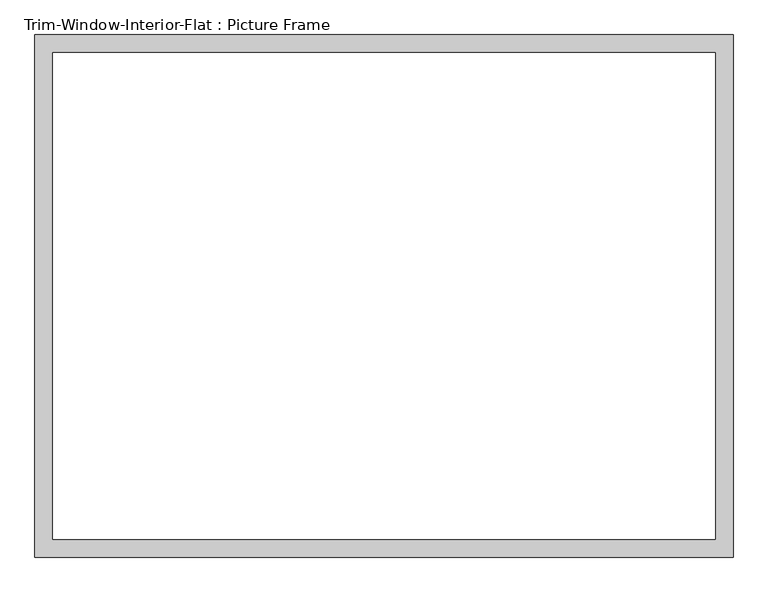
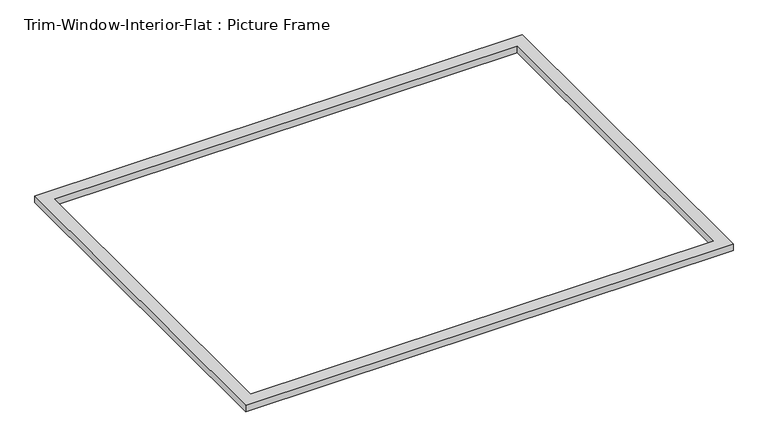
"""IFC4 building model written with IfcOpenShell, lengths in millimetres: proxy geometry, Trim-Window-Interior-Flat : Picture Frame."""

from ifc_helpers import new_model, si_unit, origin, origin_with_axes, place, context, project, spatial, polyline, outline, extrude, source, transform, mapped, element, save


def trim_window_interior_flat_picture_frame_e25f2530(model_context):
    return source(origin(), model_context, "Body", "SweptSolid", [
        extrude(outline(polyline([(1111.25, 44.45), (1111.25, -1619.25), (-1111.25, -1619.25), (-1111.25, 44.45), (1111.25, 44.45)]), holes=[polyline([(1054.1, -12.7), (-1054.1, -12.7), (-1054.1, -1562.1), (1054.1, -1562.1), (1054.1, -12.7)])]), origin_with_axes(), (0.0, 0.0, 1.0), 31.75),
    ])


if __name__ == "__main__":
    model = new_model("IFC4")
    model_context = context("Model", 3, world=origin())
    ifc_project = project(units=[si_unit("LENGTHUNIT", "METRE", prefix="MILLI")], contexts=[model_context])
    site = spatial("IfcSite", under=ifc_project)
    building = spatial("IfcBuilding", under=site)
    placement = place(None, origin())
    trim_window_interior_flat_picture_frame_shape = trim_window_interior_flat_picture_frame_e25f2530(model_context)
    element("IfcBuildingElementProxy", 1, Name="Trim-Window-Interior-Flat : Picture Frame", ObjectType="Trim-Window-Interior-Flat : Picture Frame", at=placement, inside=building, context=model_context, shape_type="MappedRepresentation", body=[
        mapped(trim_window_interior_flat_picture_frame_shape, transform((0.0, 0.0, 0.0), x_axis=(1.0, 0.0, 0.0), y_axis=(0.0, 1.0, 0.0), z_axis=(0.0, 0.0, 1.0))),
    ])
    save(model, "model.ifc")

# Revit data of these elements
# Type "Trim-Window-Interior-Flat : Picture Frame"
#   Trim Thickness_Picture Frame = 0' - 1 1/4"
#   Trim Width = 0' - 2 1/4"
#   Trim Thickness_with Sill = 0' - 0 3/4"
#   Sill Thickness = 0' - 1 1/4"
#   Opening Width [instance default] = 2' - 0"
#   Opening Height [instance default] = 3' - 0"
#   Default Elevation = 4' - 0"
#   Sill = no
#   Picture Frame = yes
#   Trim Material [instance default] = none
# Element 1 (IfcBuildingElementProxy, "Trim-Window-Interior-Flat : Picture Frame")
#   Opening Width = 7' - 0"
#   Opening Height = 5' - 2"
#   Trim Material = Wood - Stained
#   Materials on its faces: "Wood - Stained"
# Materials
#   "Wood - Stained": class "Wood", colour RGB 224 178 126, transparency 0, Cost = 0
